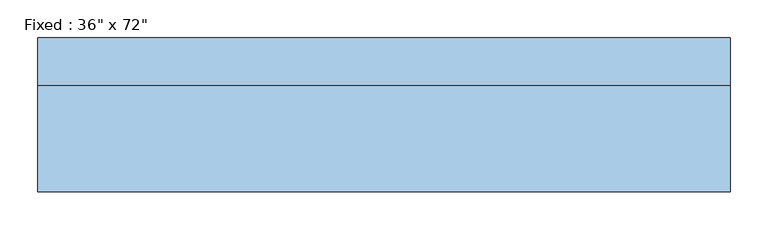
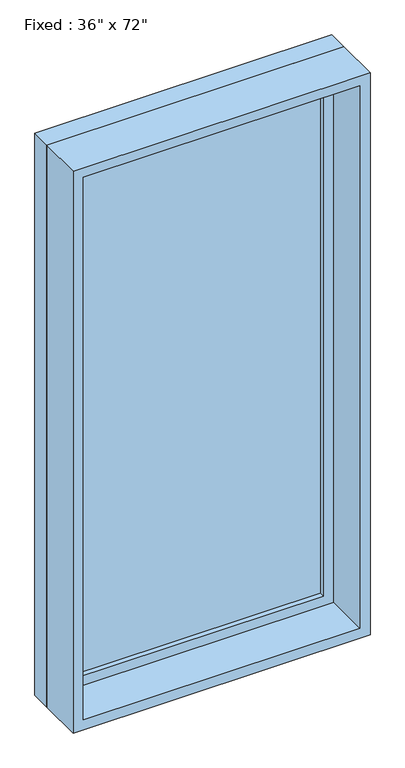
"""IFC4 building model written with IfcOpenShell, lengths in millimetres: window geometry."""

from ifc_helpers import new_model, si_unit, frame, origin, place, context, project, spatial, polyline, outline, extrude, source, transform, mapped, element, save


def window_9a779fa2(model_context):
    return source(origin(), model_context, "Body", "SweptSolid", [
        extrude(outline(polyline([(355.6, 53.975), (-431.8, 53.975), (-431.8, 66.675), (355.6, 66.675), (355.6, 53.975)])), frame((0.0, 0.0, 368.3), z_axis=(0.0, 0.0, 1.0), x_axis=(1.0, 0.0, 0.0)), (0.0, 0.0, 1.0), 1701.8),
        extrude(outline(polyline([(2114.55, -476.25), (323.85, -476.25), (323.85, 400.05), (2114.55, 400.05), (2114.55, -476.25)]), holes=[polyline([(2070.1, -431.8), (2070.1, 355.6), (368.3, 355.6), (368.3, -431.8), (2070.1, -431.8)])]), frame((0.0, 38.1, 0.0), z_axis=(0.0, 1.0, 0.0), x_axis=(0.0, 0.0, 1.0)), (0.0, 0.0, 1.0), 44.45),
        extrude(outline(polyline([(2133.6, -495.3), (304.8, -495.3), (304.8, 419.1), (2133.6, 419.1), (2133.6, -495.3)]), holes=[polyline([(2101.85, -463.55), (2101.85, 387.35), (336.55, 387.35), (336.55, -463.55), (2101.85, -463.55)])]), frame((0.0, -101.6, 0.0), z_axis=(0.0, 1.0, 0.0), x_axis=(0.0, 0.0, 1.0)), (0.0, 0.0, 1.0), 139.7),
        extrude(outline(polyline([(2133.6, 419.1), (2133.6, -495.3), (304.8, -495.3), (304.8, 419.1), (2133.6, 419.1)]), holes=[polyline([(2114.55, 400.05), (323.85, 400.05), (323.85, -476.25), (2114.55, -476.25), (2114.55, 400.05)])]), frame((0.0, 38.1, 0.0), z_axis=(0.0, 1.0, 0.0), x_axis=(0.0, 0.0, 1.0)), (0.0, 0.0, 1.0), 63.5),
    ])


if __name__ == "__main__":
    model = new_model("IFC4")
    model_context = context("Model", 3, world=origin())
    ifc_project = project(units=[si_unit("LENGTHUNIT", "METRE", prefix="MILLI")], contexts=[model_context])
    site = spatial("IfcSite", under=ifc_project)
    building = spatial("IfcBuilding", under=site)
    placement = place(None, origin())
    window_shape = window_9a779fa2(model_context)
    element("IfcWindow", 1, ObjectType="Fixed : 36\" x 72\"", at=placement, inside=building, context=model_context, shape_type="MappedRepresentation", body=[
        mapped(window_shape, transform((0.0, 0.0, 0.0), x_axis=(1.0, 0.0, 0.0), y_axis=(0.0, 1.0, 0.0), z_axis=(0.0, 0.0, 1.0))),
    ])
    save(model, "model.ifc")

# Revit data of these elements
# Type "Fixed : 36\" x 72\""
#   Type Mark = "9"
#   Construction Type Id = "GSP4R"
#   Assembly Code = "B2020100"
#   Analytic Construction = "1/8 in Pilkington single glazing"
#   Visual Light Transmittance = 0.9
#   Solar Heat Gain Coefficient = 0.78
#   Heat Transfer Coefficient (U) = 0.6496 BTU/(h·ft²·°F)
#   Height = 6' - 0"
#   Default Sill Height = 1' - 0"
#   Width = 3' - 0"
#   Window Inset = 0' - 0 3/4"
#   Define Thermal Properties by = 1
#   Glass Pane Material = Glass
#   Sash Material = Sash
#   Wall Closure = (empty or 0)
# Element 1 (IfcWindow, "Fixed : 36\" x 72\"")
#   Materials on its faces: "Sash", "Glass"
# Materials
#   "Glass": class "Glass", colour RGB 0 128 192, transparency 0.75, Description = "Soda Lime Glass", Cost = 0
#   "Sash": class "Wood", colour RGB 224 178 126, transparency 0
